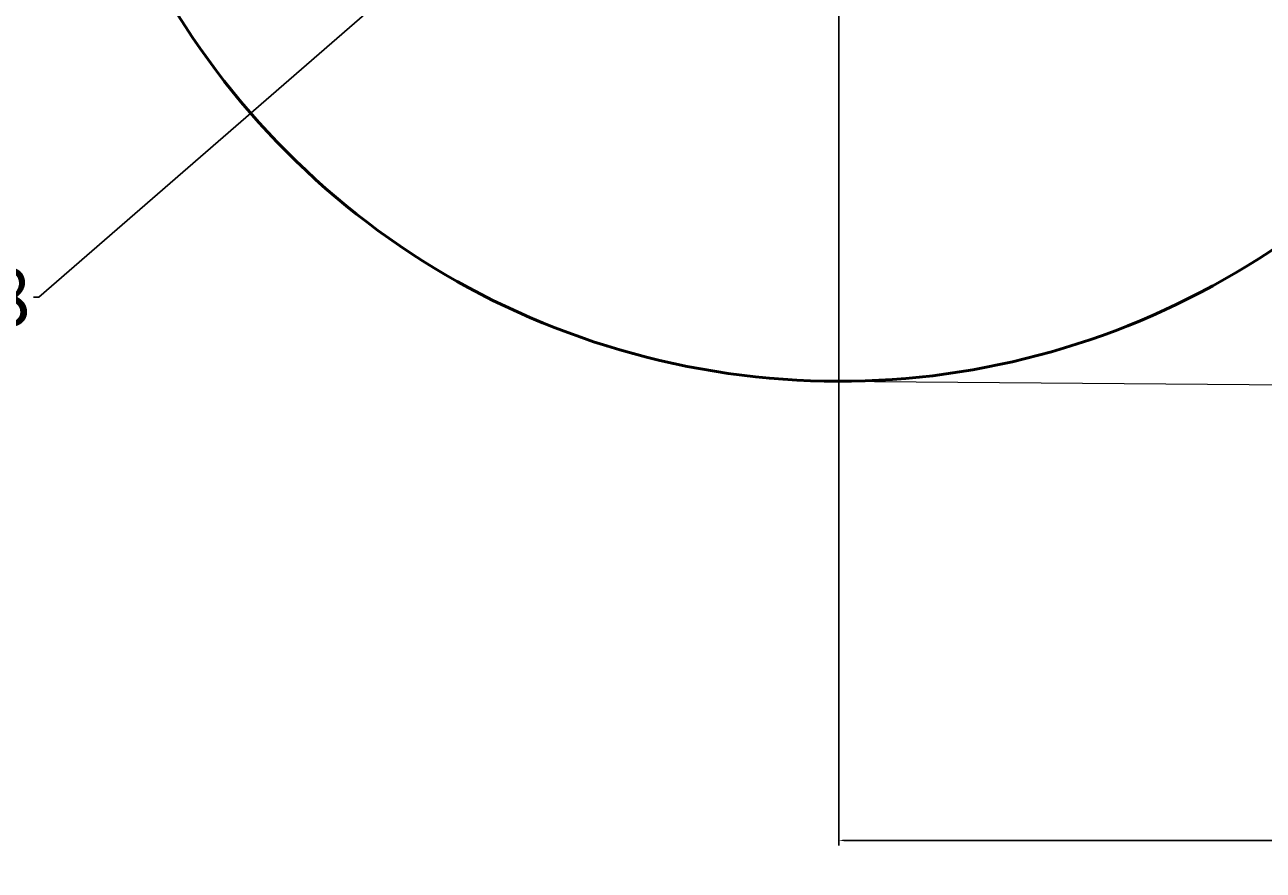
# Model space of a CAD drawing. Units: millimetres. Extents: x -60 to 113, y -37 to 126.
# Tile 2 of 17: x -21 to 22, y -37 to -8. Entities that reach past the tile are written whole.
import ezdxf

# ---------------------------------------------------------------- set-up
doc = ezdxf.new("R2010")
doc.units = ezdxf.units.MM
doc.header["$MEASUREMENT"] = 0
doc.linetypes.add('CENTER2', pattern=[1.125, 0.75, -0.125, 0.125, -0.125])
for name, color, linetype, lineweight in [('M-CNTR', 4, 'CENTER2', 18), ('M-CONS', 8, 'Continuous', 13), ('M-DIMS', 2, 'Continuous', 25), ('M-OUTL', 7, 'Continuous', 50)]:
    doc.layers.add(name, color=color, linetype=linetype, lineweight=lineweight)
doc.styles.get("Standard").update_dxf_attribs({"font": 'arial.ttf'})
doc.dimstyles.get("Standard").update_dxf_attribs({"dimtxt": 0.18, "dimasz": 0.18, "dimexe": 0.18, "dimexo": 0.0625, "dimgap": 0.09, "dimtad": 0, "dimtih": 1, "dimtoh": 1, "dimdec": 4, "dimzin": 0, "dimdsep": 46, "dimtxsty": 'Standard', "dimcen": 0.09, "dimadec": 0, "dimazin": 0, "dimtfac": 1, "dimtdec": 4, "dimtofl": 0, "dimtmove": 0, "dimatfit": 3, "dimfxl": 1, "dimtolj": 1, "dimtzin": 0, "dimarcsym": 0})

# ---------------------------------------------------------------- blocks, each defined once
blk = doc.blocks.new('*U2')
at = {"layer": 'M-CNTR', "color": 0, "transparency": 16777216}
blk.add_line((0, -27.12), (0, -5.4), dxfattribs=at)
blk = doc.blocks.new('*D14')
at = {"layer": 'Defpoints', "color": 0, "transparency": 16777216}
for p in [(7.267, 6.903), (67.355, 6.442), (67.355, -36.011)]:
    blk.add_point(p, dxfattribs=at)
at = {"layer": 'M-DIMS', "color": 0, "lineweight": -2, "transparency": 16777216}
for p, q in [((7.267, 6.84), (7.267, -36.191)), ((67.355, 6.379), (67.355, -36.191)), ((7.447, -36.011), (35.786, -36.011)), ((67.175, -36.011), (38.835, -36.011))]:
    blk.add_line(p, q, dxfattribs=at)
at = {"layer": 'M-DIMS', "color": 0, "transparency": 16777216}
for points in [[(7.447, -35.981), (7.447, -36.041), (7.267, -36.011)], [(67.175, -35.981), (67.175, -36.041), (67.355, -36.011)]]:
    blk.add_solid(points, dxfattribs=at)
at = {"layer": 'M-DIMS', "color": 0, "transparency": 16777216, "insert": (37.311, -36.011), "char_height": 0.18, "attachment_point": 5}
blk.add_mtext('\\A1;{\\H11.11111x;60}', dxfattribs=at)
blk = doc.blocks.new('*D15')
at = {"layer": 'Defpoints', "color": 0, "transparency": 16777216}
for p in [(17.836, 16.083), (-3.303, -2.278)]:
    blk.add_point(p, dxfattribs=at)
at = {"layer": 'M-DIMS', "color": 0, "lineweight": -2, "transparency": 16777216}
for p, q in [((7.177, 6.903), (7.357, 6.903)), ((7.267, 6.813), (7.267, 6.993)), ((-20.464, -17.184), (-3.439, -2.396)), ((-20.644, -17.184), (-20.464, -17.184))]:
    blk.add_line(p, q, dxfattribs=at)
at = {"layer": 'M-DIMS', "color": 0, "transparency": 16777216}
blk.add_solid([(-3.459, -2.373), (-3.419, -2.419), (-3.303, -2.278)], dxfattribs=at)
at = {"layer": 'M-DIMS', "color": 0, "transparency": 16777216, "insert": (-24.497, -17.184), "char_height": 0.18, "attachment_point": 5}
blk.add_mtext('\\A1;{\\H11.11111x;3-%%C28}', dxfattribs=at)

msp = doc.modelspace()

# ---------------------------------------------------------------- linework, layer by layer
at = {"layer": 'M-CONS'}
msp.add_line((7.05918, -20.09651), (67.05741, -20.55741), dxfattribs=at)
at = {"layer": 'M-OUTL'}
msp.add_arc((7.26659, 6.9027), 27, 131.866655, 323.73509, dxfattribs=at)

# ---------------------------------------------------------------- block references
at = {"layer": 'M-CNTR'}
msp.add_blockref('*U2', (7.26659, 6.9027), dxfattribs=at)

# ---------------------------------------------------------------- dimensions: what is measured, and where the dimension line sits
at = {"layer": 'M-DIMS'}
dim = msp.add_diameter_dim_2p(p1=(17.83613, 16.08337), p2=(-3.30296, -2.27798), text='{\\H11.11111x;3-%%C28}', dimstyle='Standard', override={"dimclrd": 0, "dimclre": 0, "dimclrt": 0}, dxfattribs=at)
dim.commit()
dim.dimension.update_dxf_attribs({"geometry": '*D15', "text_midpoint": (-24.49681, -17.18418), "dimtype": 163})
dim = msp.add_linear_dim(base=(67.35481, -36.0105), p1=(7.26659, 6.9027), p2=(67.35481, 6.44179), text='{\\H11.11111x;60}', dimstyle='Standard', override={"dimclrd": 0, "dimclre": 0, "dimclrt": 0}, dxfattribs=at)
dim.commit()
dim.dimension.update_dxf_attribs({"geometry": '*D14', "text_midpoint": (37.3107, -36.0105)})

doc.saveas('drawing.dxf')
